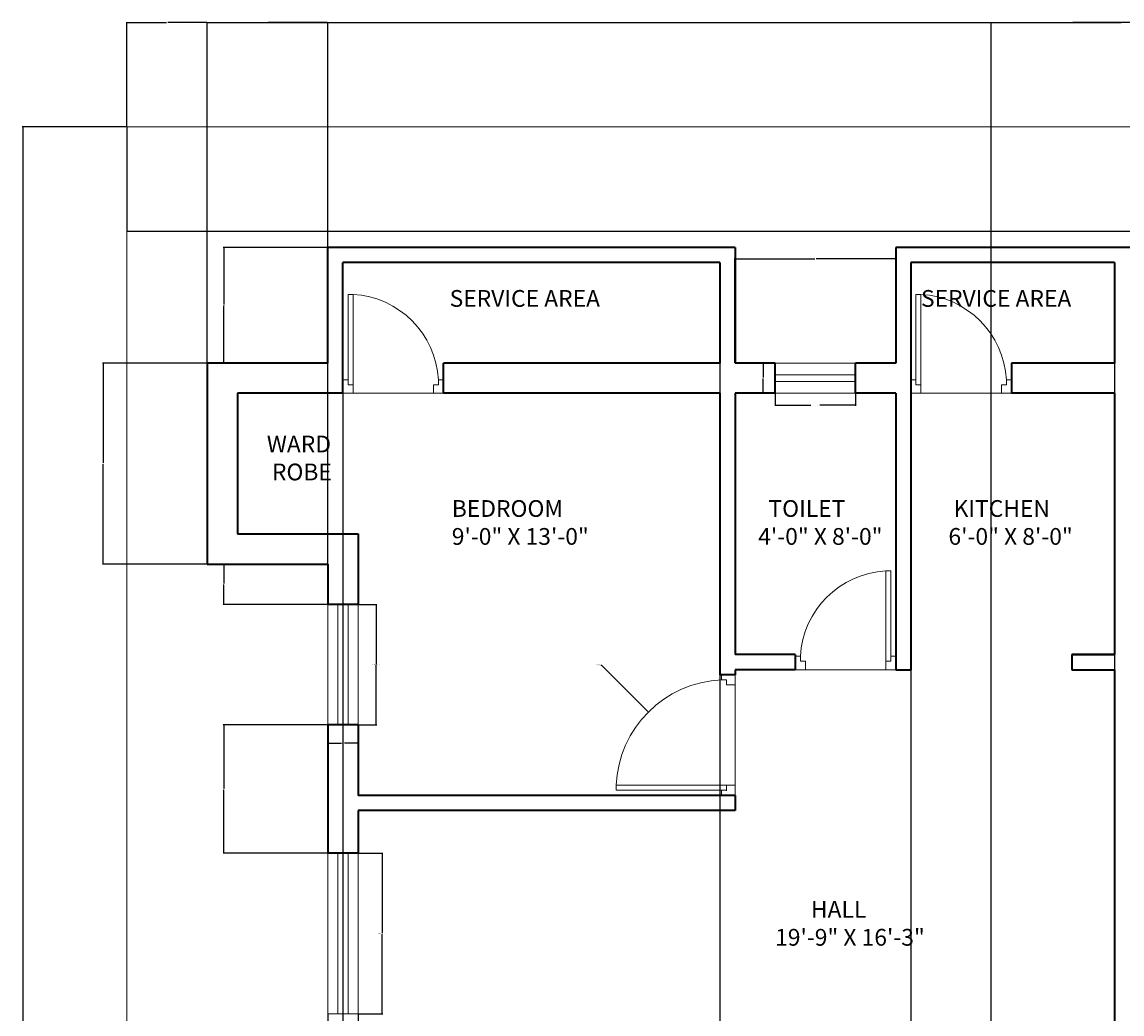
# Model space of a CAD drawing. Units: inches. Extents: x 3263 to 3926, y 954 to 1556.
# Tile 2 of 3: x 3263 to 3592, y 1260 to 1556. Entities that reach past the tile are written whole.
import ezdxf

# ---------------------------------------------------------------- set-up
doc = ezdxf.new("R2010")
doc.units = ezdxf.units.IN
for name, color, linetype, lineweight in [('A-ANNO-DIMS', 2, 'Continuous', 18), ('A-ANNO-TEXT', 7, 'Continuous', 18), ('A-AREA-IDEN', 7, 'Continuous', 18), ('C-PROP', 8, 'Continuous', 18), ('door', 30, 'Continuous', 18), ('ventilator', 210, 'Continuous', 18), ('wall', 7, 'Continuous', 35), ('window', 92, 'Continuous', 18)]:
    doc.layers.add(name, color=color, linetype=linetype, lineweight=lineweight)
doc.styles.get("Standard").update_dxf_attribs({"font": 'arial.ttf'})
doc.dimstyles.get("Standard").update_dxf_attribs({"dimtxt": 0.18, "dimasz": 0.18, "dimexe": 0.18, "dimexo": 0.0625, "dimgap": 0.09, "dimtad": 0, "dimtih": 1, "dimtoh": 1, "dimdec": 4, "dimzin": 0, "dimdsep": 46, "dimtxsty": 'Standard', "dimcen": 0.09, "dimadec": 0, "dimazin": 0, "dimtfac": 1, "dimtdec": 4, "dimtofl": 0, "dimtmove": 0, "dimatfit": 3, "dimfxl": 1, "dimtolj": 1, "dimtzin": 0, "dimarcsym": 0})

# ---------------------------------------------------------------- blocks, each defined once
blk = doc.blocks.new('d2')
at = {"layer": 'door'}
blk.add_line((4131.56, 1215.38), (4161.56, 1215.38), dxfattribs=at)
blk.add_lwpolyline([(4133.06, 1217.88), (4134.56, 1217.88), (4134.56, 1244.88), (4133.06, 1244.88)], close=True, dxfattribs=at)
for points in [[(4134.56, 1215.38), (4131.56, 1215.38), (4131.56, 1219.38), (4133.06, 1219.38), (4133.06, 1217.88), (4134.56, 1217.88), (4134.56, 1215.38)], [(4158.56, 1215.38), (4161.56, 1215.38), (4161.56, 1219.38), (4160.06, 1219.38), (4160.06, 1217.88), (4158.56, 1217.88), (4158.56, 1215.38)]]:
    blk.add_lwpolyline(points, dxfattribs=at)
blk.add_arc((4133.06, 1217.88), 27.04, 3.1798, 86.8202, dxfattribs=at)
blk = doc.blocks.new('w1')
at = {"layer": 'window'}
for p, q in [((3981.35, 1421.04), (3981.35, 1373.04)), ((3984.35, 1421.04), (3984.35, 1373.04))]:
    blk.add_line(p, q, dxfattribs=at)
blk.add_lwpolyline([(3978.35, 1373.04), (3987.35, 1373.04), (3987.35, 1421.04), (3978.35, 1421.04)], close=True, dxfattribs=at)
blk = doc.blocks.new('w2')
at = {"layer": 'window'}
for p, q in [((4050.84, 1450.41), (4050.84, 1414.41)), ((4053.84, 1450.41), (4053.84, 1414.41))]:
    blk.add_line(p, q, dxfattribs=at)
blk.add_lwpolyline([(4047.84, 1414.41), (4056.84, 1414.41), (4056.84, 1450.41), (4047.84, 1450.41)], close=True, dxfattribs=at)
blk = doc.blocks.new('d1')
at = {"layer": 'door'}
blk.add_line((4131.56, 1272.79), (4167.56, 1272.79), dxfattribs=at)
blk.add_lwpolyline([(4133.06, 1275.29), (4134.56, 1275.29), (4134.56, 1308.29), (4133.06, 1308.29)], close=True, dxfattribs=at)
for points in [[(4134.56, 1272.79), (4131.56, 1272.79), (4131.56, 1276.79), (4133.06, 1276.79), (4133.06, 1275.29), (4134.56, 1275.29), (4134.56, 1272.79)], [(4164.56, 1272.79), (4167.56, 1272.79), (4167.56, 1276.79), (4166.06, 1276.79), (4166.06, 1275.29), (4164.56, 1275.29), (4164.56, 1272.79)]]:
    blk.add_lwpolyline(points, dxfattribs=at)
blk.add_arc((4133.06, 1275.29), 33.03, 2.6026, 87.3974, dxfattribs=at)
blk = doc.blocks.new('v')
at = {"layer": 'ventilator'}
for p, q in [((4001.32, 1413.1), (4001.32, 1389.1)), ((4003.32, 1413.1), (4003.32, 1389.1))]:
    blk.add_line(p, q, dxfattribs=at)
blk.add_lwpolyline([(3997.82, 1389.1), (4006.82, 1389.1), (4006.82, 1413.1), (3997.82, 1413.1)], close=True, dxfattribs=at)
blk = doc.blocks.new('*D10')
at = {"layer": 'A-ANNO-DIMS', "color": 0, "lineweight": -2, "transparency": 16777216}
for p, q in [((3363.74, 1308.18), (3371.05, 1308.18)), ((3370.87, 1308), (3370.87, 1284.36)), ((3370.87, 1260.36), (3370.87, 1284)), ((3363.74, 1260.18), (3371.05, 1260.18))]:
    blk.add_line(p, q, dxfattribs=at)
at = {"layer": 'A-ANNO-DIMS', "color": 0, "transparency": 16777216}
for points in [[(3370.84, 1308), (3370.9, 1308), (3370.87, 1308.18)], [(3370.84, 1260.36), (3370.9, 1260.36), (3370.87, 1260.18)]]:
    blk.add_solid(points, dxfattribs=at)
at = {"layer": 'Defpoints', "color": 0, "transparency": 16777216}
for p in [(3363.67, 1308.18), (3370.87, 1308.18), (3363.67, 1260.18)]:
    blk.add_point(p, dxfattribs=at)
at = {"layer": 'A-ANNO-DIMS', "color": 0, "transparency": 16777216, "insert": (3370.87, 1284.18), "char_height": 0.18, "attachment_point": 5}
blk.add_mtext('\\A1;WINDOW W1 48 TYP.', dxfattribs=at)
blk = doc.blocks.new('*D11')
at = {"layer": 'A-ANNO-DIMS', "color": 0, "lineweight": -2, "transparency": 16777216}
for p, q in [((3354.67, 1260.12), (3354.67, 1252.8)), ((3363.67, 1260.12), (3363.67, 1252.8)), ((3354.85, 1252.98), (3358.72, 1252.98)), ((3363.49, 1252.98), (3359.63, 1252.98))]:
    blk.add_line(p, q, dxfattribs=at)
at = {"layer": 'A-ANNO-DIMS', "color": 0, "transparency": 16777216}
for points in [[(3354.85, 1253.01), (3354.85, 1252.95), (3354.67, 1252.98)], [(3363.49, 1253.01), (3363.49, 1252.95), (3363.67, 1252.98)]]:
    blk.add_solid(points, dxfattribs=at)
at = {"layer": 'Defpoints', "color": 0, "transparency": 16777216}
for p in [(3354.67, 1260.18), (3363.67, 1260.18), (3363.67, 1252.98)]:
    blk.add_point(p, dxfattribs=at)
at = {"layer": 'A-ANNO-DIMS', "color": 0, "transparency": 16777216, "insert": (3359.17, 1252.98), "char_height": 0.18, "attachment_point": 5}
blk.add_mtext('\\A1;9 TYP.', dxfattribs=at)
blk = doc.blocks.new('*D12')
at = {"layer": 'A-ANNO-DIMS', "color": 0, "lineweight": -2, "transparency": 16777216}
for p, q in [((3363.74, 1382.43), (3369.25, 1382.43)), ((3369.07, 1382.25), (3369.07, 1364.61)), ((3369.07, 1346.61), (3369.07, 1364.25)), ((3363.74, 1346.43), (3369.25, 1346.43))]:
    blk.add_line(p, q, dxfattribs=at)
at = {"layer": 'A-ANNO-DIMS', "color": 0, "transparency": 16777216}
for points in [[(3369.04, 1382.25), (3369.1, 1382.25), (3369.07, 1382.43)], [(3369.04, 1346.61), (3369.1, 1346.61), (3369.07, 1346.43)]]:
    blk.add_solid(points, dxfattribs=at)
at = {"layer": 'Defpoints', "color": 0, "transparency": 16777216}
for p in [(3363.67, 1382.43), (3369.07, 1382.43), (3363.67, 1346.43)]:
    blk.add_point(p, dxfattribs=at)
at = {"layer": 'A-ANNO-DIMS', "color": 0, "transparency": 16777216, "insert": (3369.07, 1364.43), "char_height": 0.18, "attachment_point": 5}
blk.add_mtext('\\A1;WINDOW W2 36 TYP.', dxfattribs=at)
blk = doc.blocks.new('*D13')
at = {"layer": 'A-ANNO-DIMS', "color": 0, "lineweight": -2, "transparency": 16777216}
for p, q in [((3354.67, 1346.37), (3354.67, 1340.85)), ((3363.67, 1346.37), (3363.67, 1340.85)), ((3354.85, 1341.03), (3358.72, 1341.03)), ((3363.49, 1341.03), (3359.63, 1341.03))]:
    blk.add_line(p, q, dxfattribs=at)
at = {"layer": 'A-ANNO-DIMS', "color": 0, "transparency": 16777216}
for points in [[(3354.85, 1341.06), (3354.85, 1341), (3354.67, 1341.03)], [(3363.49, 1341.06), (3363.49, 1341), (3363.67, 1341.03)]]:
    blk.add_solid(points, dxfattribs=at)
at = {"layer": 'Defpoints', "color": 0, "transparency": 16777216}
for p in [(3354.67, 1346.43), (3363.67, 1346.43), (3363.67, 1341.03)]:
    blk.add_point(p, dxfattribs=at)
at = {"layer": 'A-ANNO-DIMS', "color": 0, "transparency": 16777216, "insert": (3359.17, 1341.03), "char_height": 0.18, "attachment_point": 5}
blk.add_mtext('\\A1;9 TYP.', dxfattribs=at)
blk = doc.blocks.new('*D14')
at = {"layer": 'A-ANNO-DIMS', "color": 0, "lineweight": -2, "transparency": 16777216}
for p, q in [((3488.17, 1445.37), (3488.17, 1441.65)), ((3512.17, 1445.37), (3512.17, 1441.65)), ((3488.35, 1441.83), (3498.82, 1441.83)), ((3511.99, 1441.83), (3501.53, 1441.83))]:
    blk.add_line(p, q, dxfattribs=at)
at = {"layer": 'A-ANNO-DIMS', "color": 0, "transparency": 16777216}
for points in [[(3488.35, 1441.86), (3488.35, 1441.8), (3488.17, 1441.83)], [(3511.99, 1441.86), (3511.99, 1441.8), (3512.17, 1441.83)]]:
    blk.add_solid(points, dxfattribs=at)
at = {"layer": 'Defpoints', "color": 0, "transparency": 16777216}
for p in [(3488.17, 1445.43), (3512.17, 1445.43), (3512.17, 1441.83)]:
    blk.add_point(p, dxfattribs=at)
at = {"layer": 'A-ANNO-DIMS', "color": 0, "transparency": 16777216, "insert": (3500.17, 1441.83), "char_height": 0.18, "attachment_point": 5}
blk.add_mtext('\\A1;VENTILATOR 24 TYP.', dxfattribs=at)
blk = doc.blocks.new('*D15')
at = {"layer": 'A-ANNO-DIMS', "color": 0, "lineweight": -2, "transparency": 16777216}
for p, q in [((3488.11, 1454.43), (3484.39, 1454.43)), ((3484.57, 1454.25), (3484.57, 1450.11)), ((3484.57, 1445.61), (3484.57, 1449.75)), ((3488.11, 1445.43), (3484.39, 1445.43))]:
    blk.add_line(p, q, dxfattribs=at)
at = {"layer": 'A-ANNO-DIMS', "color": 0, "transparency": 16777216}
for points in [[(3484.54, 1454.25), (3484.6, 1454.25), (3484.57, 1454.43)], [(3484.54, 1445.61), (3484.6, 1445.61), (3484.57, 1445.43)]]:
    blk.add_solid(points, dxfattribs=at)
at = {"layer": 'Defpoints', "color": 0, "transparency": 16777216}
for p in [(3488.17, 1454.43), (3484.57, 1445.43), (3488.17, 1445.43)]:
    blk.add_point(p, dxfattribs=at)
at = {"layer": 'A-ANNO-DIMS', "color": 0, "transparency": 16777216, "insert": (3484.57, 1449.93), "char_height": 0.18, "attachment_point": 5}
blk.add_mtext('\\A1;9 TYP.', dxfattribs=at)
blk = doc.blocks.new('*D16')
at = {"layer": 'A-ANNO-DIMS', "color": 0, "lineweight": -2, "transparency": 16777216}
for p, q in [((3294.67, 1524.87), (3294.67, 1493.65)), ((3894.67, 1524.87), (3894.67, 1493.65)), ((3294.85, 1493.83), (3594.39, 1493.83)), ((3894.49, 1493.83), (3594.96, 1493.83))]:
    blk.add_line(p, q, dxfattribs=at)
at = {"layer": 'A-ANNO-DIMS', "color": 0, "transparency": 16777216}
for points in [[(3294.85, 1493.86), (3294.85, 1493.8), (3294.67, 1493.83)], [(3894.49, 1493.86), (3894.49, 1493.8), (3894.67, 1493.83)]]:
    blk.add_solid(points, dxfattribs=at)
at = {"layer": 'Defpoints', "color": 0, "transparency": 16777216}
for p in [(3294.67, 1524.93), (3894.67, 1524.93), (3294.67, 1493.83)]:
    blk.add_point(p, dxfattribs=at)
at = {"layer": 'A-ANNO-DIMS', "color": 0, "transparency": 16777216, "insert": (3594.67, 1493.83), "char_height": 0.18, "attachment_point": 5}
blk.add_mtext('\\A1;600', dxfattribs=at)
blk = doc.blocks.new('*D17')
at = {"layer": 'A-ANNO-DIMS', "color": 0, "lineweight": -2, "transparency": 16777216}
for p, q in [((3294.61, 1524.93), (3263.39, 1524.93)), ((3263.57, 1524.75), (3263.57, 1255.11)), ((3263.57, 985.11), (3263.57, 1254.75)), ((3294.61, 984.93), (3263.39, 984.93))]:
    blk.add_line(p, q, dxfattribs=at)
at = {"layer": 'A-ANNO-DIMS', "color": 0, "transparency": 16777216}
for points in [[(3263.54, 1524.75), (3263.6, 1524.75), (3263.57, 1524.93)], [(3263.54, 985.11), (3263.6, 985.11), (3263.57, 984.93)]]:
    blk.add_solid(points, dxfattribs=at)
at = {"layer": 'Defpoints', "color": 0, "transparency": 16777216}
for p in [(3263.57, 1524.93), (3294.67, 1524.93), (3294.67, 984.93)]:
    blk.add_point(p, dxfattribs=at)
at = {"layer": 'A-ANNO-DIMS', "color": 0, "transparency": 16777216, "insert": (3263.57, 1254.93), "char_height": 0.18, "attachment_point": 5}
blk.add_mtext('\\A1;540', dxfattribs=at)
blk = doc.blocks.new('*D18')
at = {"layer": 'A-ANNO-DIMS', "color": 0, "lineweight": -2, "transparency": 16777216}
for p, q in [((3294.67, 1524.99), (3294.67, 1556.21)), ((3318.67, 1454.49), (3318.67, 1556.21)), ((3294.85, 1556.03), (3306.45, 1556.03)), ((3318.49, 1556.03), (3306.89, 1556.03))]:
    blk.add_line(p, q, dxfattribs=at)
at = {"layer": 'A-ANNO-DIMS', "color": 0, "transparency": 16777216}
for points in [[(3294.85, 1556.06), (3294.85, 1556), (3294.67, 1556.03)], [(3318.49, 1556.06), (3318.49, 1556), (3318.67, 1556.03)]]:
    blk.add_solid(points, dxfattribs=at)
at = {"layer": 'Defpoints', "color": 0, "transparency": 16777216}
for p in [(3318.67, 1556.03), (3294.67, 1524.93), (3318.67, 1454.43)]:
    blk.add_point(p, dxfattribs=at)
at = {"layer": 'A-ANNO-DIMS', "color": 0, "transparency": 16777216, "insert": (3306.67, 1556.03), "char_height": 0.18, "attachment_point": 5}
blk.add_mtext('\\A1;24', dxfattribs=at)
blk = doc.blocks.new('*D19')
at = {"layer": 'A-ANNO-DIMS', "color": 0, "lineweight": -2, "transparency": 16777216}
for p, q in [((3318.67, 1454.49), (3318.67, 1556.21)), ((3834.67, 1488.99), (3834.67, 1556.21)), ((3318.85, 1556.03), (3576.39, 1556.03)), ((3834.49, 1556.03), (3576.96, 1556.03))]:
    blk.add_line(p, q, dxfattribs=at)
at = {"layer": 'A-ANNO-DIMS', "color": 0, "transparency": 16777216}
for points in [[(3318.85, 1556.06), (3318.85, 1556), (3318.67, 1556.03)], [(3834.49, 1556.06), (3834.49, 1556), (3834.67, 1556.03)]]:
    blk.add_solid(points, dxfattribs=at)
at = {"layer": 'Defpoints', "color": 0, "transparency": 16777216}
for p in [(3834.67, 1556.03), (3834.67, 1488.93), (3318.67, 1454.43)]:
    blk.add_point(p, dxfattribs=at)
at = {"layer": 'A-ANNO-DIMS', "color": 0, "transparency": 16777216, "insert": (3576.67, 1556.03), "char_height": 0.18, "attachment_point": 5}
blk.add_mtext('\\A1;516', dxfattribs=at)
blk = doc.blocks.new('*D29')
at = {"layer": 'A-ANNO-DIMS', "color": 0, "lineweight": -2, "transparency": 16777216}
for p, q in [((3552.67, 1020.99), (3552.67, 1556.21)), ((3630.67, 1020.99), (3630.67, 1556.21)), ((3552.85, 1556.03), (3591.46, 1556.03)), ((3630.49, 1556.03), (3591.89, 1556.03))]:
    blk.add_line(p, q, dxfattribs=at)
at = {"layer": 'A-ANNO-DIMS', "color": 0, "transparency": 16777216}
for points in [[(3552.85, 1556.06), (3552.85, 1556), (3552.67, 1556.03)], [(3630.49, 1556.06), (3630.49, 1556), (3630.67, 1556.03)]]:
    blk.add_solid(points, dxfattribs=at)
at = {"layer": 'Defpoints', "color": 0, "transparency": 16777216}
for p in [(3630.67, 1556.03), (3552.67, 1020.93), (3630.67, 1020.93)]:
    blk.add_point(p, dxfattribs=at)
at = {"layer": 'A-ANNO-DIMS', "color": 0, "transparency": 16777216, "insert": (3591.67, 1556.03), "char_height": 0.18, "attachment_point": 5}
blk.add_mtext('\\A1;78', dxfattribs=at)
blk = doc.blocks.new('*D33')
at = {"layer": 'A-ANNO-DIMS', "color": 0, "lineweight": -2, "transparency": 16777216}
for p, q in [((3318.67, 1394.49), (3318.67, 1556.21)), ((3354.67, 1394.49), (3354.67, 1556.21)), ((3318.85, 1556.03), (3336.46, 1556.03)), ((3354.49, 1556.03), (3336.89, 1556.03))]:
    blk.add_line(p, q, dxfattribs=at)
at = {"layer": 'A-ANNO-DIMS', "color": 0, "transparency": 16777216}
for points in [[(3318.85, 1556.06), (3318.85, 1556), (3318.67, 1556.03)], [(3354.49, 1556.06), (3354.49, 1556), (3354.67, 1556.03)]]:
    blk.add_solid(points, dxfattribs=at)
at = {"layer": 'Defpoints', "color": 0, "transparency": 16777216}
for p in [(3354.67, 1556.03), (3318.67, 1394.43), (3354.67, 1394.43)]:
    blk.add_point(p, dxfattribs=at)
at = {"layer": 'A-ANNO-DIMS', "color": 0, "transparency": 16777216, "insert": (3336.67, 1556.03), "char_height": 0.18, "attachment_point": 5}
blk.add_mtext('\\A1;36', dxfattribs=at)
blk = doc.blocks.new('*D34')
at = {"layer": 'A-ANNO-DIMS', "color": 0, "lineweight": -2, "transparency": 16777216}
for p, q in [((3318.61, 1454.43), (3287.39, 1454.43)), ((3287.57, 1454.25), (3287.57, 1424.61)), ((3287.57, 1394.61), (3287.57, 1424.25)), ((3318.61, 1394.43), (3287.39, 1394.43))]:
    blk.add_line(p, q, dxfattribs=at)
at = {"layer": 'A-ANNO-DIMS', "color": 0, "transparency": 16777216}
for points in [[(3287.54, 1454.25), (3287.6, 1454.25), (3287.57, 1454.43)], [(3287.54, 1394.61), (3287.6, 1394.61), (3287.57, 1394.43)]]:
    blk.add_solid(points, dxfattribs=at)
at = {"layer": 'Defpoints', "color": 0, "transparency": 16777216}
for p in [(3287.57, 1454.43), (3318.67, 1454.43), (3318.67, 1394.43)]:
    blk.add_point(p, dxfattribs=at)
at = {"layer": 'A-ANNO-DIMS', "color": 0, "transparency": 16777216, "insert": (3287.57, 1424.43), "char_height": 0.18, "attachment_point": 5}
blk.add_mtext('\\A1;60', dxfattribs=at)
blk = doc.blocks.new('*D35')
at = {"layer": 'A-ANNO-DIMS', "color": 0, "lineweight": -2, "transparency": 16777216}
for p, q in [((3354.61, 1488.93), (3323.39, 1488.93)), ((3323.57, 1488.75), (3323.57, 1471.86)), ((3323.57, 1454.61), (3323.57, 1471.5)), ((3354.61, 1454.43), (3323.39, 1454.43))]:
    blk.add_line(p, q, dxfattribs=at)
at = {"layer": 'A-ANNO-DIMS', "color": 0, "transparency": 16777216}
for points in [[(3323.54, 1488.75), (3323.6, 1488.75), (3323.57, 1488.93)], [(3323.54, 1454.61), (3323.6, 1454.61), (3323.57, 1454.43)]]:
    blk.add_solid(points, dxfattribs=at)
at = {"layer": 'Defpoints', "color": 0, "transparency": 16777216}
for p in [(3323.57, 1488.93), (3354.67, 1488.93), (3354.67, 1454.43)]:
    blk.add_point(p, dxfattribs=at)
at = {"layer": 'A-ANNO-DIMS', "color": 0, "transparency": 16777216, "insert": (3323.57, 1471.68), "char_height": 0.18, "attachment_point": 5}
blk.add_mtext('\\A1;34.5', dxfattribs=at)
blk = doc.blocks.new('*D36')
at = {"layer": 'A-ANNO-DIMS', "color": 0, "lineweight": -2, "transparency": 16777216}
for p, q in [((3359.17, 1484.37), (3359.17, 953.65)), ((3471.67, 1484.37), (3471.67, 953.65)), ((3359.35, 953.83), (3415.04, 953.83)), ((3471.49, 953.83), (3415.81, 953.83))]:
    blk.add_line(p, q, dxfattribs=at)
at = {"layer": 'A-ANNO-DIMS', "color": 0, "transparency": 16777216}
for points in [[(3359.35, 953.86), (3359.35, 953.8), (3359.17, 953.83)], [(3471.49, 953.86), (3471.49, 953.8), (3471.67, 953.83)]]:
    blk.add_solid(points, dxfattribs=at)
at = {"layer": 'Defpoints', "color": 0, "transparency": 16777216}
for p in [(3359.17, 1484.43), (3471.67, 1484.43), (3471.67, 953.83)]:
    blk.add_point(p, dxfattribs=at)
at = {"layer": 'A-ANNO-DIMS', "color": 0, "transparency": 16777216, "insert": (3415.42, 953.83), "char_height": 0.18, "attachment_point": 5}
blk.add_mtext('\\A1;112.5', dxfattribs=at)
blk = doc.blocks.new('*D37')
at = {"layer": 'A-ANNO-DIMS', "color": 0, "lineweight": -2, "transparency": 16777216}
for p, q in [((3476.17, 1454.49), (3476.17, 1485.71)), ((3476.35, 1485.53), (3499.95, 1485.53)), ((3523.99, 1485.53), (3500.4, 1485.53)), ((3524.17, 1454.49), (3524.17, 1485.71))]:
    blk.add_line(p, q, dxfattribs=at)
at = {"layer": 'A-ANNO-DIMS', "color": 0, "transparency": 16777216}
for points in [[(3476.35, 1485.56), (3476.35, 1485.5), (3476.17, 1485.53)], [(3523.99, 1485.56), (3523.99, 1485.5), (3524.17, 1485.53)]]:
    blk.add_solid(points, dxfattribs=at)
at = {"layer": 'Defpoints', "color": 0, "transparency": 16777216}
for p in [(3524.17, 1485.53), (3476.17, 1454.43), (3524.17, 1454.43)]:
    blk.add_point(p, dxfattribs=at)
at = {"layer": 'A-ANNO-DIMS', "color": 0, "transparency": 16777216, "insert": (3500.17, 1485.53), "char_height": 0.18, "attachment_point": 5}
blk.add_mtext('\\A1;48', dxfattribs=at)
blk = doc.blocks.new('*D38')
at = {"layer": 'A-ANNO-DIMS', "color": 0, "lineweight": -2, "transparency": 16777216}
for p, q in [((3528.67, 1484.37), (3528.67, 953.65)), ((3589.42, 1484.37), (3589.42, 953.65)), ((3528.85, 953.83), (3558.65, 953.83)), ((3589.24, 953.83), (3559.44, 953.83))]:
    blk.add_line(p, q, dxfattribs=at)
at = {"layer": 'A-ANNO-DIMS', "color": 0, "transparency": 16777216}
for points in [[(3528.85, 953.86), (3528.85, 953.8), (3528.67, 953.83)], [(3589.24, 953.86), (3589.24, 953.8), (3589.42, 953.83)]]:
    blk.add_solid(points, dxfattribs=at)
at = {"layer": 'Defpoints', "color": 0, "transparency": 16777216}
for p in [(3528.67, 1484.43), (3589.42, 1484.43), (3589.42, 953.83)]:
    blk.add_point(p, dxfattribs=at)
at = {"layer": 'A-ANNO-DIMS', "color": 0, "transparency": 16777216, "insert": (3559.05, 953.83), "char_height": 0.18, "attachment_point": 5}
blk.add_mtext('\\A1;60.75', dxfattribs=at)
blk = doc.blocks.new('*D47')
at = {"layer": 'A-ANNO-DIMS', "color": 0, "lineweight": -2, "transparency": 16777216}
for p, q in [((3354.61, 1394.43), (3323.39, 1394.43)), ((3323.57, 1394.25), (3323.57, 1388.61)), ((3323.57, 1382.61), (3323.57, 1388.25)), ((3354.61, 1382.43), (3323.39, 1382.43))]:
    blk.add_line(p, q, dxfattribs=at)
at = {"layer": 'A-ANNO-DIMS', "color": 0, "transparency": 16777216}
for points in [[(3323.54, 1394.25), (3323.6, 1394.25), (3323.57, 1394.43)], [(3323.54, 1382.61), (3323.6, 1382.61), (3323.57, 1382.43)]]:
    blk.add_solid(points, dxfattribs=at)
at = {"layer": 'Defpoints', "color": 0, "transparency": 16777216}
for p in [(3323.57, 1394.43), (3354.67, 1394.43), (3354.67, 1382.43)]:
    blk.add_point(p, dxfattribs=at)
at = {"layer": 'A-ANNO-DIMS', "color": 0, "transparency": 16777216, "insert": (3323.57, 1388.43), "char_height": 0.18, "attachment_point": 5}
blk.add_mtext('\\A1;12', dxfattribs=at)
blk = doc.blocks.new('*D48')
at = {"layer": 'A-ANNO-DIMS', "color": 0, "lineweight": -2, "transparency": 16777216}
for p, q in [((3354.61, 1346.43), (3323.39, 1346.43)), ((3323.57, 1346.25), (3323.57, 1327.49)), ((3323.57, 1308.36), (3323.57, 1327.12)), ((3354.61, 1308.18), (3323.39, 1308.18))]:
    blk.add_line(p, q, dxfattribs=at)
at = {"layer": 'A-ANNO-DIMS', "color": 0, "transparency": 16777216}
for points in [[(3323.54, 1346.25), (3323.6, 1346.25), (3323.57, 1346.43)], [(3323.54, 1308.36), (3323.6, 1308.36), (3323.57, 1308.18)]]:
    blk.add_solid(points, dxfattribs=at)
at = {"layer": 'Defpoints', "color": 0, "transparency": 16777216}
for p in [(3323.57, 1346.43), (3354.67, 1346.43), (3354.67, 1308.18)]:
    blk.add_point(p, dxfattribs=at)
at = {"layer": 'A-ANNO-DIMS', "color": 0, "transparency": 16777216, "insert": (3323.57, 1327.31), "char_height": 0.18, "attachment_point": 5}
blk.add_mtext('\\A1;38.25', dxfattribs=at)
blk = doc.blocks.new('*D58')
at = {"layer": 'A-ANNO-DIMS', "color": 0, "lineweight": -2, "transparency": 16777216}
for p, q in [((3436.12, 1364.3), (3436.3, 1364.3)), ((3436.3, 1364.3), (3450.19, 1350.42)), ((3473.58, 1326.93), (3473.76, 1326.93)), ((3473.67, 1326.84), (3473.67, 1327.02))]:
    blk.add_line(p, q, dxfattribs=at)
at = {"layer": 'A-ANNO-DIMS', "color": 0, "transparency": 16777216}
blk.add_solid([(3450.21, 1350.44), (3450.17, 1350.4), (3450.32, 1350.29)], dxfattribs=at)
at = {"layer": 'Defpoints', "color": 0, "transparency": 16777216}
for p in [(3450.32, 1350.29), (3473.67, 1326.93)]:
    blk.add_point(p, dxfattribs=at)
at = {"layer": 'A-ANNO-DIMS', "color": 0, "transparency": 16777216, "insert": (3435.38, 1364.3), "char_height": 0.18, "attachment_point": 5}
blk.add_mtext('\\A1;6X R33.034', dxfattribs=at)

msp = doc.modelspace()

# ---------------------------------------------------------------- linework, layer by layer
at = {"layer": 'C-PROP'}
for p, q in [((3894.6743, 1524.9303), (3294.6743, 1524.9303)), ((3294.6743, 1524.9303), (3294.6743, 984.9303))]:
    msp.add_line(p, q, dxfattribs=at)
at = {"layer": 'wall'}
for p, q in [((3476.1743, 1488.9303), (3354.6743, 1488.9303)), ((3354.6743, 1454.4303), (3354.6743, 1488.9303)), ((3476.1743, 1488.9303), (3476.1743, 1454.4303)), ((3834.6743, 1488.9303), (3524.1743, 1488.9303)), ((3524.1743, 1488.9303), (3524.1743, 1454.4303)), ((3471.6743, 1484.4303), (3359.1743, 1484.4303)), ((3359.1743, 1445.4303), (3359.1743, 1484.4303)), ((3471.6743, 1484.4303), (3471.6743, 1454.4303)), ((3528.6743, 1484.4303), (3528.6743, 1445.4303)), ((3589.4243, 1484.4303), (3528.6743, 1484.4303)), ((3589.4243, 1484.4303), (3589.4243, 1454.4303)), ((3354.6743, 1454.4303), (3318.6743, 1454.4303)), ((3318.6743, 1454.4303), (3318.6743, 1394.4303)), ((3389.1743, 1445.4303), (3389.1743, 1454.4303)), ((3471.6743, 1454.4303), (3389.1743, 1454.4303)), ((3488.1743, 1454.4303), (3476.1743, 1454.4303)), ((3488.1743, 1445.4303), (3488.1743, 1454.4303)), ((3524.1743, 1454.4303), (3512.1743, 1454.4303)), ((3512.1743, 1445.4303), (3512.1743, 1454.4303)), ((3558.6743, 1454.4303), (3558.6743, 1445.4303)), ((3589.4243, 1454.4303), (3558.6743, 1454.4303)), ((3359.1743, 1445.4303), (3327.6743, 1445.4303)), ((3327.6743, 1445.4303), (3327.6743, 1403.4303)), ((3359.1743, 1445.4303), (3354.6743, 1445.4303)), ((3471.6743, 1445.4303), (3389.1743, 1445.4303)), ((3471.6743, 1445.4303), (3471.6743, 1361.4303)), ((3476.1743, 1445.4303), (3476.1743, 1367.4303)), ((3488.1743, 1445.4303), (3476.1743, 1445.4303)), ((3524.1743, 1445.4303), (3512.1743, 1445.4303)), ((3524.1743, 1445.4303), (3524.1743, 1362.9303)), ((3528.6743, 1445.4303), (3528.6743, 1362.9303)), ((3589.4243, 1445.4303), (3558.6743, 1445.4303)), ((3589.4243, 1445.4303), (3589.4243, 1367.4303)), ((3327.6743, 1403.4303), (3363.6743, 1403.4303)), ((3363.6743, 1403.4303), (3363.6743, 1382.4303)), ((3318.6743, 1394.4303), (3354.6743, 1394.4303)), ((3354.6743, 1394.4303), (3354.6743, 1382.4303)), ((3363.6743, 1382.4303), (3354.6743, 1382.4303)), ((3494.1743, 1367.4303), (3476.1743, 1367.4303)), ((3494.1743, 1367.4303), (3494.1743, 1362.9303)), ((3589.4243, 1367.4303), (3576.6743, 1367.4303)), ((3576.6743, 1367.4303), (3576.6743, 1362.9303)), ((3576.6743, 1367.4303), (3589.4243, 1367.4303)), ((3494.1743, 1362.9303), (3476.1743, 1362.9303)), ((3476.1743, 1362.9303), (3476.1743, 1361.4303)), ((3524.1743, 1362.9303), (3528.6743, 1362.9303)), ((3576.6743, 1362.9303), (3589.4243, 1362.9303)), ((3589.4243, 1362.9303), (3589.4243, 1194.9303)), ((3476.1743, 1361.4303), (3471.6743, 1361.4303)), ((3363.6743, 1346.4303), (3354.6743, 1346.4303)), ((3354.6743, 1346.4303), (3354.6743, 1308.1803)), ((3363.6743, 1346.4303), (3363.6743, 1325.4303)), ((3476.1743, 1325.4303), (3363.6743, 1325.4303)), ((3476.1743, 1325.4303), (3476.1743, 1320.9303)), ((3476.1743, 1320.9303), (3363.6743, 1320.9303)), ((3363.6743, 1320.9303), (3363.6743, 1308.1803)), ((3363.6743, 1308.1803), (3354.6743, 1308.1803))]:
    msp.add_line(p, q, dxfattribs=at)

# ---------------------------------------------------------------- block references
at = {"layer": 'door'}
for p in [(-772.3842, 230.0526), (-602.8842, 230.0526)]:
    msp.add_blockref('d2', p, dxfattribs=at)
at = {"layer": 'door', "xscale": -1}
msp.add_blockref('d2', (7655.7328, 147.5526), dxfattribs=at)
at = {"layer": 'door', "rotation": 90.00000000000003}
msp.add_blockref('d1', (4748.9614, -2806.1282), dxfattribs=at)
at = {"layer": 'ventilator', "rotation": 270}
msp.add_blockref('v', (2099.0732, 5452.2479), dxfattribs=at)
at = {"layer": 'window'}
for name, p in [('w2', (-693.1644, -67.9784)), ('w1', (-623.6806, -112.8567))]:
    msp.add_blockref(name, p, dxfattribs=at)

# ---------------------------------------------------------------- texts
at = {"layer": 'A-ANNO-TEXT', "insert": (3336.4362, 1432.7629), "char_height": 5, "attachment_point": 1}
msp.add_mtext_dynamic_manual_height_columns('WARD   ROBE', width=21.465717, gutter_width=12.5, heights=[0], dxfattribs=at)
at = {"layer": 'A-AREA-IDEN', "char_height": 5, "attachment_point": 1}
for s, width, insert in [('SERVICE AREA', 62.092631, (3390.9994, 1476.2215)), ('SERVICE AREA', 62.092631, (3531.6743, 1476.2215)), ('BEDROOM\\P9\'-0" X 13\'-0"', 42.17852, (3391.6415, 1413.5302)), ('  TOILET\\P4\'-0" X 8\'-0"', 42.17852, (3483.0982, 1413.5302)), (' KITCHEN\\P6\'-0" X 8\'-0"', 42.17852, (3539.8783, 1413.5302)), ('       HALL\\P19\'-9" X 16\'-3"', 69.358735, (3488.1397, 1293.9022))]:
    msp.add_mtext_dynamic_manual_height_columns(s, width=width, gutter_width=12.5, heights=[0], dxfattribs=dict(at, insert=insert))

# ---------------------------------------------------------------- dimensions: what is measured, and where the dimension line sits
at = {"layer": 'A-ANNO-DIMS'}
for base, p1, p2, override, picture, middle in [((3318.6743, 1556.0303), (3294.6743, 1524.9303), (3318.6743, 1454.4303), {"dimdec": 0, "dimlfac": 1, "dimrnd": 0, "dimzin": 0, "dimdsep": 46, "dimlunit": 2}, '*D18', (3306.6743, 1556.0303)), ((3834.6743, 1556.0303), (3318.6743, 1454.4303), (3834.6743, 1488.9303), {"dimdec": 0, "dimlfac": 1, "dimrnd": 0, "dimzin": 0, "dimdsep": 46, "dimlunit": 2}, '*D19', (3576.6743, 1556.0303)), ((3354.6743, 1556.0303), (3318.6743, 1394.4303), (3354.6743, 1394.4303), {"dimdec": 0, "dimlfac": 1, "dimrnd": 0, "dimzin": 0, "dimdsep": 46, "dimlunit": 2}, '*D33', (3336.6743, 1556.0303)), ((3630.6743, 1556.0303), (3552.6743, 1020.9303), (3630.6743, 1020.9303), {"dimdec": 0, "dimlfac": 1, "dimrnd": 0, "dimzin": 0, "dimdsep": 46, "dimlunit": 2}, '*D29', (3591.6743, 1556.0303)), ((3471.6743, 953.8303), (3359.1743, 1484.4303), (3471.6743, 1484.4303), {"dimdec": 1, "dimlfac": 1, "dimrnd": 0, "dimzin": 0, "dimdsep": 46, "dimlunit": 2}, '*D36', (3415.4243, 953.8303)), ((3524.1743, 1485.5303), (3476.1743, 1454.4303), (3524.1743, 1454.4303), {"dimdec": 0, "dimlfac": 1, "dimrnd": 0, "dimzin": 0, "dimdsep": 46, "dimlunit": 2}, '*D37', (3500.1743, 1485.5303)), ((3589.4243, 953.8303), (3528.6743, 1484.4303), (3589.4243, 1484.4303), {"dimdec": 2, "dimlfac": 1, "dimrnd": 0, "dimzin": 0, "dimdsep": 46, "dimlunit": 2}, '*D38', (3559.0493, 953.8303))]:
    dim = msp.add_linear_dim(base=base, p1=p1, p2=p2, dimstyle='Standard', override=override, dxfattribs=at)
    dim.commit()
    dim.dimension.update_dxf_attribs({"geometry": picture, "text_midpoint": middle})
for base, p1, p2, angle, override, picture, middle in [((3263.5743, 1524.9303), (3294.6743, 984.9303), (3294.6743, 1524.9303), 90, {"dimdec": 0, "dimlfac": 1, "dimrnd": 0, "dimzin": 0, "dimdsep": 46, "dimlunit": 2}, '*D17', (3263.5743, 1254.9303)), ((3294.6743, 1493.8303), (3894.6743, 1524.9303), (3294.6743, 1524.9303), 180, {"dimdec": 0, "dimlfac": 1, "dimrnd": 0, "dimzin": 0, "dimdsep": 46, "dimlunit": 2}, '*D16', (3594.6743, 1493.8303)), ((3323.5743, 1488.9303), (3354.6743, 1454.4303), (3354.6743, 1488.9303), 90, {"dimdec": 1, "dimlfac": 1, "dimrnd": 0, "dimzin": 0, "dimdsep": 46, "dimlunit": 2}, '*D35', (3323.5743, 1471.6803)), ((3287.5743, 1454.4303), (3318.6743, 1394.4303), (3318.6743, 1454.4303), 90, {"dimdec": 0, "dimlfac": 1, "dimrnd": 0, "dimzin": 0, "dimdsep": 46, "dimlunit": 2}, '*D34', (3287.5743, 1424.4303)), ((3323.5743, 1394.4303), (3354.6743, 1382.4303), (3354.6743, 1394.4303), 90, {"dimdec": 0, "dimlfac": 1, "dimrnd": 0, "dimzin": 0, "dimdsep": 46, "dimlunit": 2}, '*D47', (3323.5743, 1388.4303)), ((3323.5743, 1346.4303), (3354.6743, 1308.1803), (3354.6743, 1346.4303), 90, {"dimdec": 2, "dimlfac": 1, "dimrnd": 0, "dimzin": 0, "dimdsep": 46, "dimlunit": 2}, '*D48', (3323.5743, 1327.3053))]:
    dim = msp.add_linear_dim(base=base, p1=p1, p2=p2, angle=angle, dimstyle='Standard', override=override, dxfattribs=at)
    dim.commit()
    dim.dimension.update_dxf_attribs({"geometry": picture, "text_midpoint": middle})
for base, p1, p2, angle, text, picture, middle in [((3484.5743, 1445.4303), (3488.1743, 1454.4303), (3488.1743, 1445.4303), 270, '<> TYP.', '*D15', (3484.5743, 1449.9303)), ((3369.0743, 1382.4303), (3363.6743, 1346.4303), (3363.6743, 1382.4303), 90, 'WINDOW W2 <> TYP.', '*D12', (3369.0743, 1364.4303)), ((3370.8743, 1308.1803), (3363.6743, 1260.1803), (3363.6743, 1308.1803), 90, 'WINDOW W1 <> TYP.', '*D10', (3370.8743, 1284.1803))]:
    dim = msp.add_linear_dim(base=base, p1=p1, p2=p2, angle=angle, text=text, dimstyle='Standard', override={"dimdec": 0, "dimlfac": 1, "dimrnd": 0, "dimzin": 0, "dimdsep": 46, "dimlunit": 2}, dxfattribs=at)
    dim.commit()
    dim.dimension.update_dxf_attribs({"geometry": picture, "text_midpoint": middle})
for base, p1, p2, text, picture, middle in [((3512.1743, 1441.8303), (3488.1743, 1445.4303), (3512.1743, 1445.4303), 'VENTILATOR <> TYP.', '*D14', (3500.1743, 1441.8303)), ((3363.6743, 1341.0303), (3354.6743, 1346.4303), (3363.6743, 1346.4303), '<> TYP.', '*D13', (3359.1743, 1341.0303)), ((3363.6743, 1252.9803), (3354.6743, 1260.1803), (3363.6743, 1260.1803), '<> TYP.', '*D11', (3359.1743, 1252.9803))]:
    dim = msp.add_linear_dim(base=base, p1=p1, p2=p2, text=text, dimstyle='Standard', override={"dimdec": 0, "dimlfac": 1, "dimrnd": 0, "dimzin": 0, "dimdsep": 46, "dimlunit": 2}, dxfattribs=at)
    dim.commit()
    dim.dimension.update_dxf_attribs({"geometry": picture, "text_midpoint": middle})
dim = msp.add_radius_dim(center=(3473.6743, 1326.9303), mpoint=(3450.3159, 1350.2891), text='6X <>', dimstyle='Standard', override={"dimdec": 3, "dimlfac": 1, "dimrnd": 0, "dimzin": 0, "dimdsep": 46, "dimlunit": 2}, dxfattribs=at)
dim.commit()
dim.dimension.update_dxf_attribs({"geometry": '*D58', "text_midpoint": (3435.3775, 1364.3044), "dimtype": 164})

doc.saveas('drawing.dxf')
